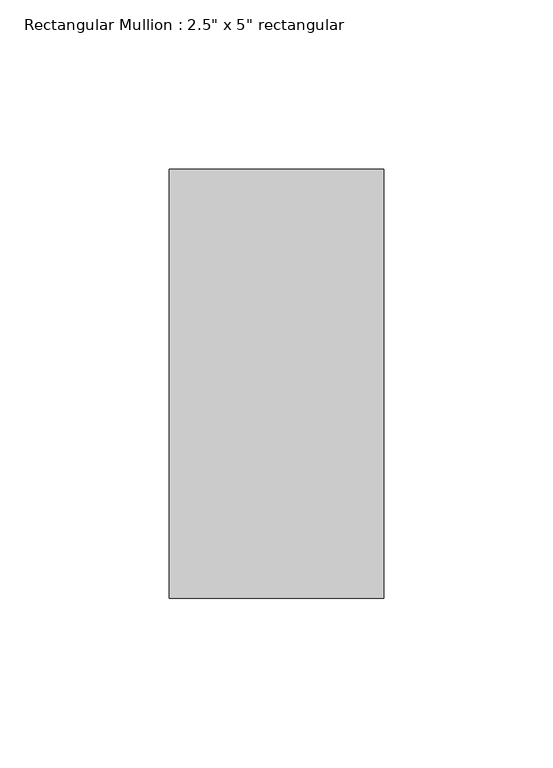
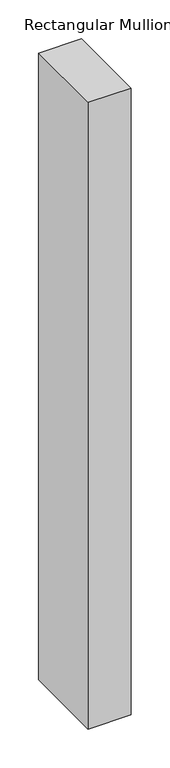
"""IFC4 building model written with IfcOpenShell, lengths in millimetres: member geometry."""

from ifc_helpers import new_model, si_unit, frame, origin, place, context, project, spatial, polyline, outline, extrude, source, transform, mapped, element, save


def member_389f1ce1(model_context):
    return source(origin(), model_context, "Body", "SweptSolid", [
        extrude(outline(polyline([(31.75, 63.5), (31.75, -63.5), (-31.75, -63.5), (-31.75, 63.5), (31.75, 63.5)])), frame((0.0, 0.0, -982.6547408), z_axis=(0.0, 0.0, 1.0), x_axis=(1.0, 0.0, 0.0)), (0.0, 0.0, 1.0), 982.6547408),
    ])


if __name__ == "__main__":
    model = new_model("IFC4")
    model_context = context("Model", 3, world=origin())
    ifc_project = project(units=[si_unit("LENGTHUNIT", "METRE", prefix="MILLI")], contexts=[model_context])
    site = spatial("IfcSite", under=ifc_project)
    building = spatial("IfcBuilding", under=site)
    placement = place(None, origin())
    member_shape = member_389f1ce1(model_context)
    element("IfcMember", 1, ObjectType="Rectangular Mullion : 2.5\" x 5\" rectangular", at=placement, inside=building, context=model_context, shape_type="MappedRepresentation", body=[
        mapped(member_shape, transform((0.0, 0.0, 0.0), x_axis=(1.0, 0.0, 0.0), y_axis=(0.0, 1.0, 0.0), z_axis=(0.0, 0.0, 1.0))),
    ])
    save(model, "model.ifc")

# Revit data of these elements
# Type "Rectangular Mullion : 2.5\" x 5\" rectangular"
#   built-in parameter 1007304 = 0.416667 (stored number, unit not read)
#   built-in parameter 1007301 = 0.104167 (stored number, unit not read)
#   built-in parameter 1007300 = 0.104167 (stored number, unit not read)
